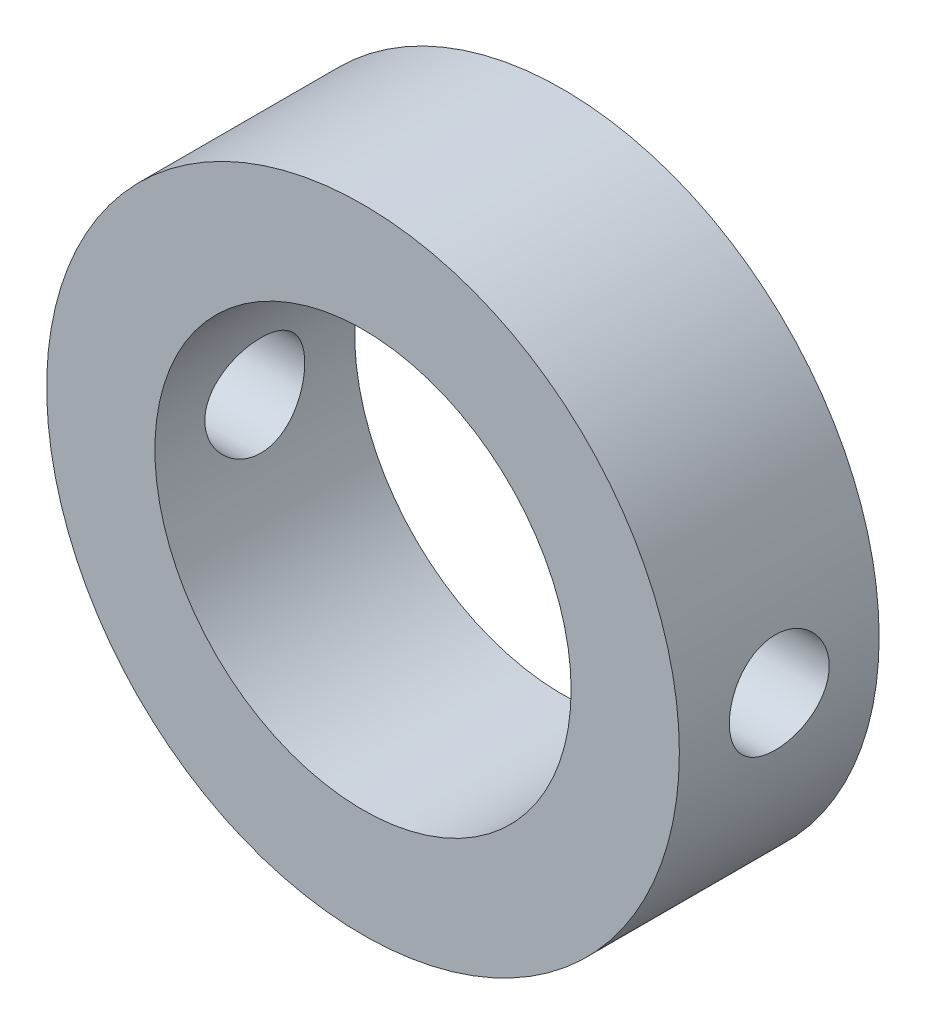
from build123d import *

# Parameters (mm, degrees)
COLLAR_RING_PROFILE_R       = 19
COLLAR_RING_PROFILE_R_2     = 12.5
COLLAR_RING_38X_25X12_DEPTH = 12
CROSS_HOLE_6_DEPTH          = 30.427877939
CROSS_HOLE_6_DEPTH_BACK     = 30.427877939
CROSS_HOLE_PROFILE_R        = 3


with BuildPart() as part:
    # Collar Ring Profile → Collar Ring Ø38xØ25x12 (new body)
    with BuildSketch(Plane.XY):
        Circle(COLLAR_RING_PROFILE_R)
        Circle(COLLAR_RING_PROFILE_R_2, mode=Mode.SUBTRACT)
    extrude(amount=COLLAR_RING_38X_25X12_DEPTH)

    # Cross Hole Profile → Cross Hole Ø6 (cut, two sides: drawn at the far end of the back side and taken through both)
    with BuildSketch(Plane(origin=(0, 0, 0), x_dir=(0, 0, -1), z_dir=(1, 0, 0)).offset(-CROSS_HOLE_6_DEPTH_BACK)):
        with Locations((-6, 0)):
            Circle(CROSS_HOLE_PROFILE_R)
    extrude(amount=CROSS_HOLE_6_DEPTH + CROSS_HOLE_6_DEPTH_BACK, mode=Mode.SUBTRACT)


solid = part.part
